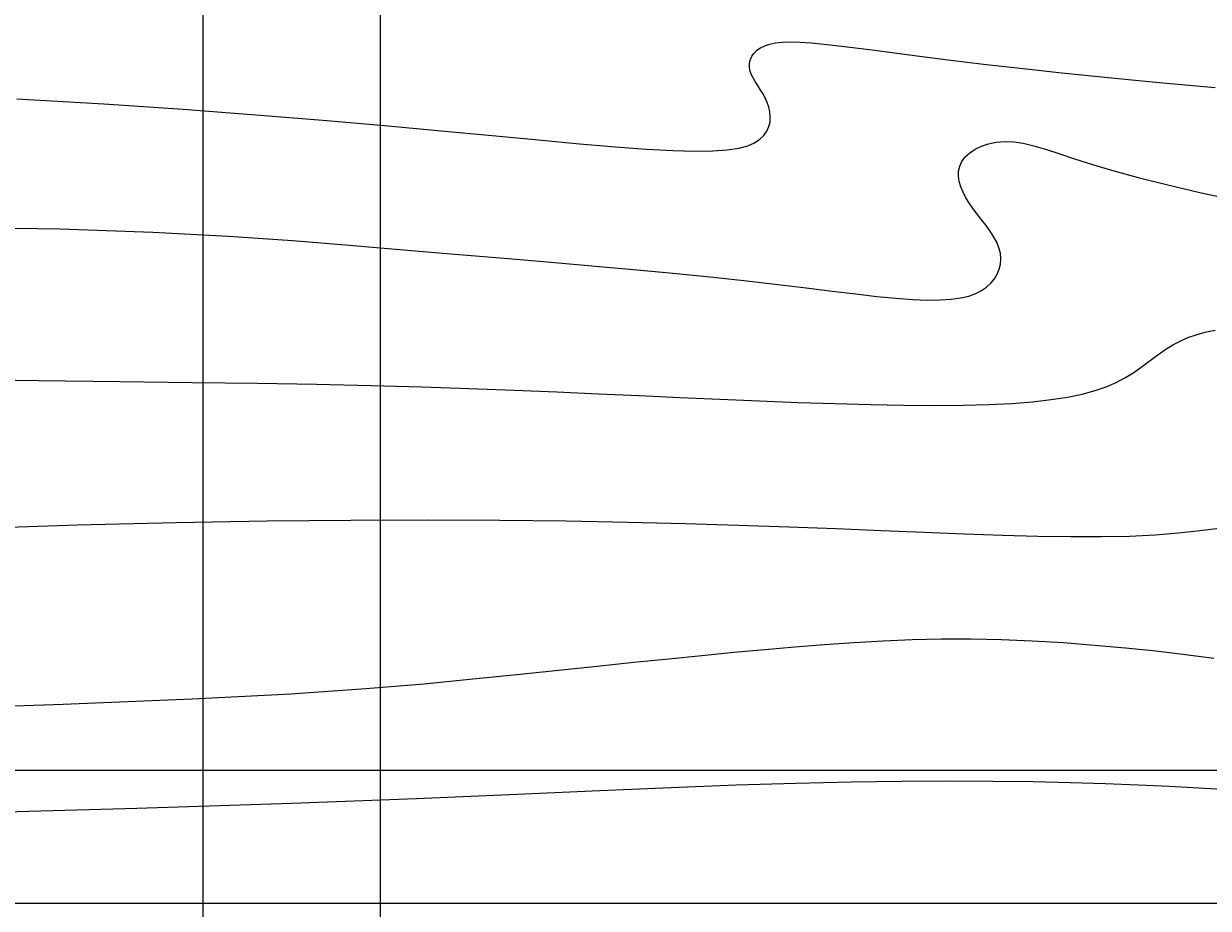
# Model space of a CAD drawing. Units: inches. Extents: x 7359 to 7979, y 33027 to 34263.
# Tile 9 of 32: x 7688 to 7728, y 33386 to 33416. Entities that reach past the tile are written whole.
import ezdxf

# ---------------------------------------------------------------- set-up
doc = ezdxf.new("R2010")
doc.units = ezdxf.units.IN
doc.layers.add('A-ANNO-DIMS', color=2, linetype='Continuous', lineweight=18)
doc.layers.add('A-FURN', color=8, linetype='Continuous', lineweight=18)
doc.styles.get("Standard").update_dxf_attribs({"font": 'arial.ttf'})
doc.dimstyles.get("Standard").update_dxf_attribs({"dimtxt": 0.18, "dimasz": 0.18, "dimexe": 0.18, "dimexo": 0.0625, "dimgap": 0.09, "dimtad": 0, "dimtih": 1, "dimtoh": 1, "dimdec": 4, "dimzin": 0, "dimdsep": 46, "dimtxsty": 'Standard', "dimcen": 0.09, "dimadec": 0, "dimazin": 0, "dimtfac": 1, "dimtdec": 4, "dimtofl": 0, "dimtmove": 0, "dimatfit": 3, "dimfxl": 1, "dimtolj": 1, "dimtzin": 0, "dimarcsym": 0})

# ---------------------------------------------------------------- blocks, each defined once
blk = doc.blocks.new('Dining Set - 36 x 72 in.')
for points in [[(-16.0362, 14.53613), (-13.0957, 14.36718), (-10.4159, 14.18652), (-7.9583, 14), (-5.6904, 13.81315), (-3.6035, 13.63021), (-1.6954, 13.45508), (0.0365, 13.29166), (1.5945, 13.14388), (2.9811, 13.01562), (4.1988, 12.9108), (5.25, 12.83333), (6.1393, 12.78613), (6.8802, 12.76823), (7.4883, 12.77767), (7.9792, 12.8125), (8.3685, 12.87077), (8.6719, 12.95052), (8.9049, 13.0498), (9.0833, 13.16666), (9.2205, 13.29899), (9.3216, 13.44401), (9.3895, 13.59879), (9.4271, 13.76041), (9.4373, 13.92594), (9.4232, 14.09245), (9.3875, 14.257), (9.3333, 14.41666), (9.2638, 14.56917), (9.1836, 14.71484), (9.0975, 14.85465), (9.0104, 14.98958), (8.9272, 15.1206), (8.8529, 15.2487), (8.7922, 15.37483), (8.75, 15.5), (8.7305, 15.62467), (8.7344, 15.74739), (8.7617, 15.86621), (8.8125, 15.97916), (8.8867, 16.08431), (8.9844, 16.17968), (9.1055, 16.26334), (9.25, 16.33333), (9.4189, 16.38802), (9.6172, 16.42708), (9.8506, 16.45052), (10.125, 16.45833), (10.4463, 16.45052), (10.8203, 16.42708), (11.2529, 16.38802), (11.75, 16.33333), (12.3184, 16.26318), (12.9694, 16.17838), (13.7151, 16.07991), (14.5677, 15.96875), (15.5395, 15.84586), (16.6426, 15.71224), (17.8893, 15.56884), (19.2917, 15.41666), (20.859, 15.25667), (22.5879, 15.08984), (24.4721, 14.91715)], [(-18.4241, 10.19775), (-14.5677, 10.13541), (-11.4399, 10.03011), (-8.877, 9.89453), (-6.7154, 9.74137), (-4.7917, 9.58333), (-2.9698, 9.43082), (-1.2246, 9.28515), (0.4415, 9.14534), (2.026, 9.01041), (3.5266, 8.87939), (4.9408, 8.7513), (6.266, 8.62516), (7.5, 8.5), (8.6411, 8.37549), (9.6914, 8.2539), (10.6538, 8.13818), (11.5312, 8.03125), (12.3267, 7.93603), (13.043, 7.85547), (13.6831, 7.79248), (14.25, 7.75), (14.7471, 7.7303), (15.1797, 7.73307), (15.5537, 7.75732), (15.875, 7.80208), (16.1494, 7.86637), (16.3828, 7.94922), (16.5811, 8.04964), (16.75, 8.16666), (16.8944, 8.29915), (17.0143, 8.44531), (17.1089, 8.60319), (17.1771, 8.77083), (17.218, 8.94629), (17.2305, 9.1276), (17.2137, 9.31282), (17.1667, 9.5), (17.0895, 9.6875), (16.987, 9.875), (16.8649, 10.0625), (16.7292, 10.25), (16.5856, 10.4375), (16.4401, 10.625), (16.2985, 10.8125), (16.1667, 11), (16.05, 11.18733), (15.9518, 11.3737), (15.8752, 11.5581), (15.8229, 11.73958), (15.798, 11.91715), (15.8034, 12.08984), (15.842, 12.25667), (15.9167, 12.41666), (16.0295, 12.56836), (16.1784, 12.70833), (16.3605, 12.83268), (16.5729, 12.9375), (16.8127, 13.01888), (17.0768, 13.07291), (17.3625, 13.0957), (17.6667, 13.08333), (17.9894, 13.03312), (18.3418, 12.94726), (18.7382, 12.82918), (19.1927, 12.68229), (19.7195, 12.51001), (20.3327, 12.31575), (21.0465, 12.10294), (21.875, 11.875), (22.8357, 11.63354), (23.959, 11.37304), (25.2786, 11.08618)], [(-18.4271, 5.05208), (-15.3009, 5.00602), (-12.5508, 4.97265), (-10.1112, 4.94515), (-7.9167, 4.91666), (-5.909, 4.88167), (-4.0586, 4.83984), (-2.3429, 4.79215), (-0.7396, 4.73958), (0.7739, 4.6831), (2.22, 4.6237), (3.6213, 4.56233), (5, 4.5), (6.373, 4.43782), (7.7344, 4.3776), (9.0723, 4.32129), (10.375, 4.27083), (11.6309, 4.22819), (12.8281, 4.19531), (13.9551, 4.17415), (15, 4.16666), (15.954, 4.17448), (16.819, 4.19791), (17.6001, 4.23698), (18.3021, 4.29166), (18.9299, 4.36198), (19.4883, 4.44791), (19.9823, 4.54948), (20.4167, 4.66666), (20.7969, 4.79899), (21.1302, 4.94401), (21.4245, 5.09879), (21.6875, 5.26041), (21.9271, 5.42594), (22.1511, 5.59245), (22.3672, 5.757), (22.5834, 5.91666), (22.8065, 6.06868), (23.0404, 6.21093), (23.2879, 6.34147), (23.5521, 6.45833), (23.8358, 6.55957), (24.142, 6.64323), (24.4735, 6.70735)], [(-17.6563, 0.00521), (-14.0005, 0.12833), (-10.6523, 0.21289), (-7.5796, 0.26522), (-4.75, 0.29166), (-2.134, 0.29793), (0.2878, 0.28711), (2.5317, 0.26163), (4.6146, 0.22396), (6.5529, 0.17651), (8.3633, 0.12174), (10.0623, 0.06209), (11.6667, 0), (13.1899, -0.06201), (14.6341, -0.1211), (15.9982, -0.17432), (17.2813, -0.21875), (18.4823, -0.25147), (19.6003, -0.26953), (20.6343, -0.27002), (21.5834, -0.25), (22.4481, -0.20768), (23.2357, -0.14584), (23.9549, -0.06836), (24.6146, 0.02083)], [(-20.084, -6.1263), (-14.469, -5.9419), (-10.1094, -5.76042), (-6.7752, -5.58285), (-4.2363, -5.41016), (-2.2629, -5.24333), (-0.625, -5.08334), (0.8708, -4.93099), (2.2715, -4.78646), (3.5872, -4.64974), (4.8281, -4.52084), (6.0046, -4.39974), (7.127, -4.28646), (8.2053, -4.18099), (9.25, -4.08334), (10.2705, -3.99382), (11.2734, -3.91407), (12.2647, -3.84603), (13.25, -3.79167), (14.2354, -3.75293), (15.2266, -3.73177), (16.2295, -3.73015), (17.25, -3.75), (18.2912, -3.79248), (19.3451, -3.85547), (20.4009, -3.93604), (21.4479, -4.03125), (22.4754, -4.13819), (23.4727, -4.25391), (24.4289, -4.37549)], [(-18.4675, -9.62891), (-11.9839, -9.45069), (-6.7396, -9.28125), (-2.5226, -9.12354), (0.8789, -8.98047), (3.6769, -8.85498), (6.0833, -8.75), (8.2767, -8.66765), (10.3021, -8.60677), (12.1712, -8.56543), (13.8958, -8.54167), (15.4876, -8.53353), (16.9583, -8.53907), (18.3197, -8.55632), (19.5834, -8.58334), (20.7616, -8.61841), (21.8685, -8.66081), (22.9188, -8.71004), (23.9271, -8.76563), (24.9081, -8.82707)]]:
    blk.add_lwpolyline(points)
blk = doc.blocks.new('*D85')
at = {"layer": 'A-ANNO-DIMS', "color": 0, "lineweight": -2, "transparency": 16777216}
for p, q in [((7793.064, 33390.662), (7369.542, 33390.662)), ((7369.722, 33390.482), (7369.722, 33388.594)), ((7369.722, 33386.342), (7369.722, 33388.231)), ((7793.064, 33386.162), (7369.542, 33386.162))]:
    blk.add_line(p, q, dxfattribs=at)
at = {"layer": 'A-ANNO-DIMS', "color": 0, "transparency": 16777216}
for points in [[(7369.692, 33390.482), (7369.752, 33390.482), (7369.722, 33390.662)], [(7369.692, 33386.342), (7369.752, 33386.342), (7369.722, 33386.162)]]:
    blk.add_solid(points, dxfattribs=at)
at = {"layer": 'Defpoints', "color": 0, "transparency": 16777216}
for p in [(7793.127, 33390.662), (7369.722, 33386.162), (7793.127, 33386.162)]:
    blk.add_point(p, dxfattribs=at)
at = {"layer": 'A-ANNO-DIMS', "color": 0, "transparency": 16777216, "insert": (7369.722, 33388.412), "char_height": 0.18, "attachment_point": 5}
blk.add_mtext('\\A1;4.5', dxfattribs=at)
blk = doc.blocks.new('*D89')
at = {"layer": 'A-ANNO-DIMS', "color": 0, "lineweight": -2, "transparency": 16777216}
for p, q in [((7693.626578, 33301.124789), (7693.626578, 33657.242289)), ((7699.626578, 33301.124789), (7699.626578, 33657.242289)), ((7693.806578, 33657.062289), (7696.477151, 33657.062289)), ((7699.446578, 33657.062289), (7696.776005, 33657.062289))]:
    blk.add_line(p, q, dxfattribs=at)
at = {"layer": 'A-ANNO-DIMS', "color": 0, "transparency": 16777216}
for points in [[(7693.806578, 33657.092289), (7693.806578, 33657.032289), (7693.626578, 33657.062289)], [(7699.446578, 33657.092289), (7699.446578, 33657.032289), (7699.626578, 33657.062289)]]:
    blk.add_solid(points, dxfattribs=at)
at = {"layer": 'Defpoints', "color": 0, "transparency": 16777216}
for p in [(7699.626578, 33657.062289), (7693.626578, 33301.062289), (7699.626578, 33301.062289)]:
    blk.add_point(p, dxfattribs=at)
at = {"layer": 'A-ANNO-DIMS', "color": 0, "transparency": 16777216, "insert": (7696.626578, 33657.062289), "char_height": 0.18, "attachment_point": 5}
blk.add_mtext('\\A1;6', dxfattribs=at)

msp = doc.modelspace()

# ---------------------------------------------------------------- block references
at = {"layer": 'A-FURN'}
msp.add_blockref('Dining Set - 36 x 72 in.', (7703.363, 33398.8436), dxfattribs=at)

# ---------------------------------------------------------------- dimensions: what is measured, and where the dimension line sits
at = {"layer": 'A-ANNO-DIMS'}
dim = msp.add_linear_dim(base=(7699.6266, 33657.0623), p1=(7693.6266, 33301.0623), p2=(7699.6266, 33301.0623), dimstyle='Standard', override={"dimdec": 0, "dimlfac": 1, "dimrnd": 0, "dimzin": 0, "dimdsep": 46, "dimlunit": 2}, dxfattribs=at)
dim.commit()
dim.dimension.update_dxf_attribs({"geometry": '*D89', "text_midpoint": (7696.6266, 33657.0623)})
dim = msp.add_linear_dim(base=(7369.7217, 33386.1623), p1=(7793.1266, 33390.6623), p2=(7793.1266, 33386.1623), angle=90, dimstyle='Standard', override={"dimdec": 1, "dimlfac": 1, "dimrnd": 0, "dimzin": 0, "dimdsep": 46, "dimlunit": 2}, dxfattribs=at)
dim.commit()
dim.dimension.update_dxf_attribs({"geometry": '*D85', "text_midpoint": (7369.7217, 33388.4123)})

doc.saveas('drawing.dxf')
